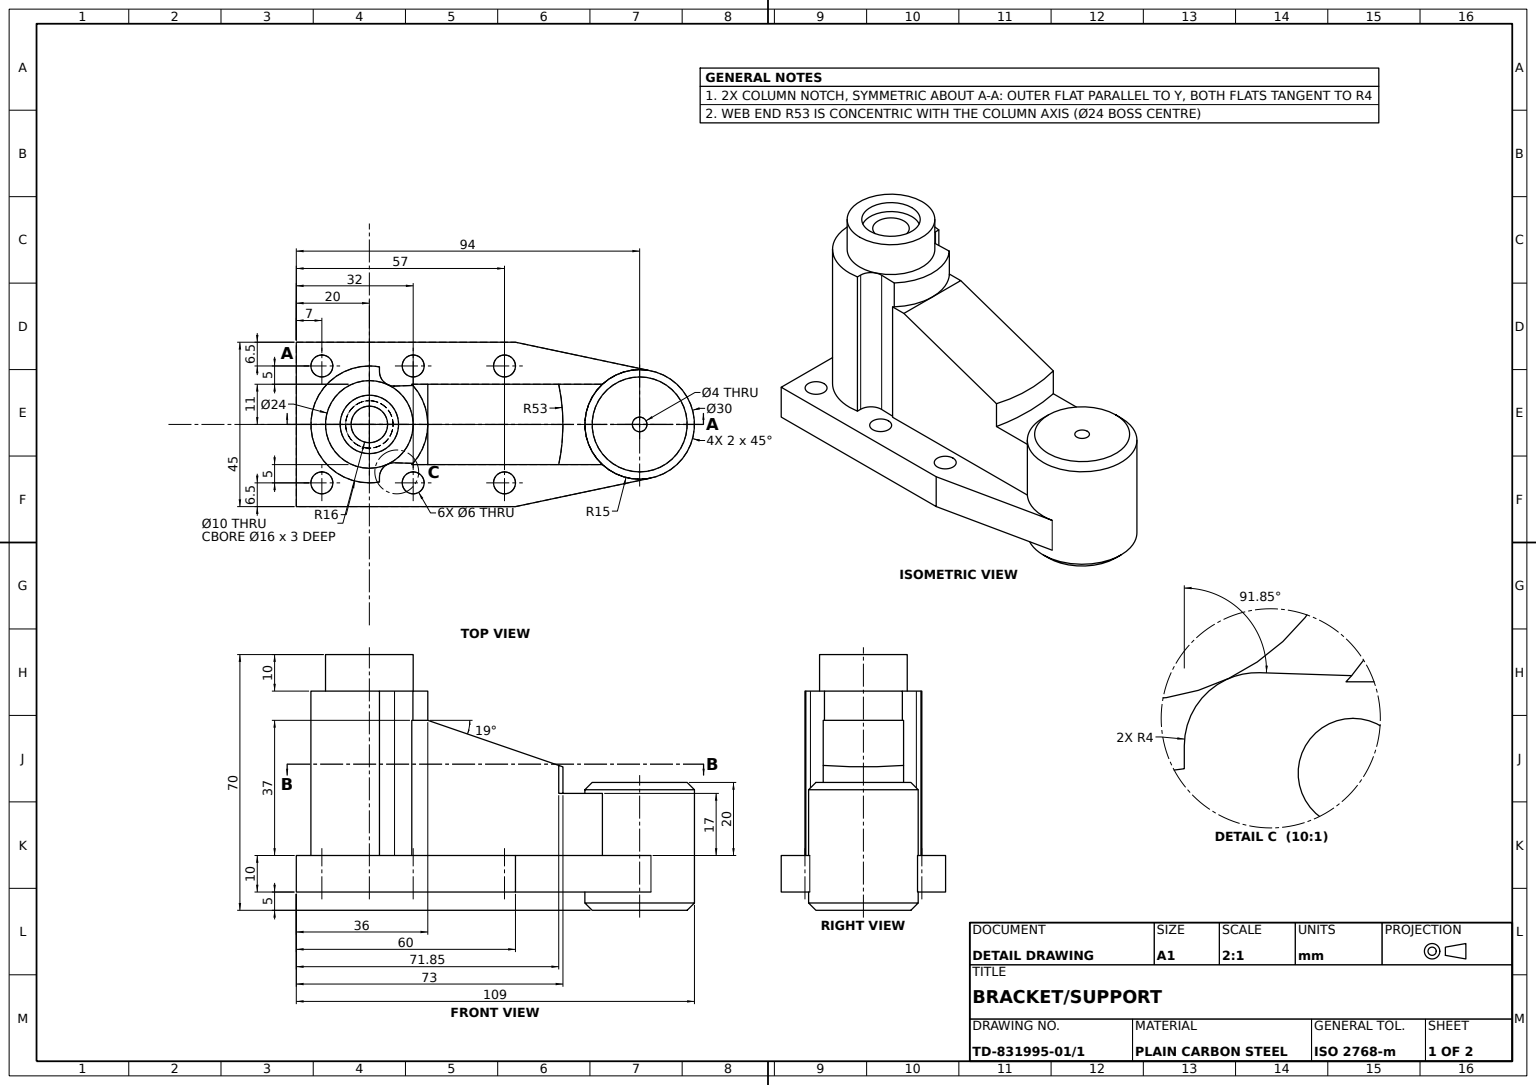
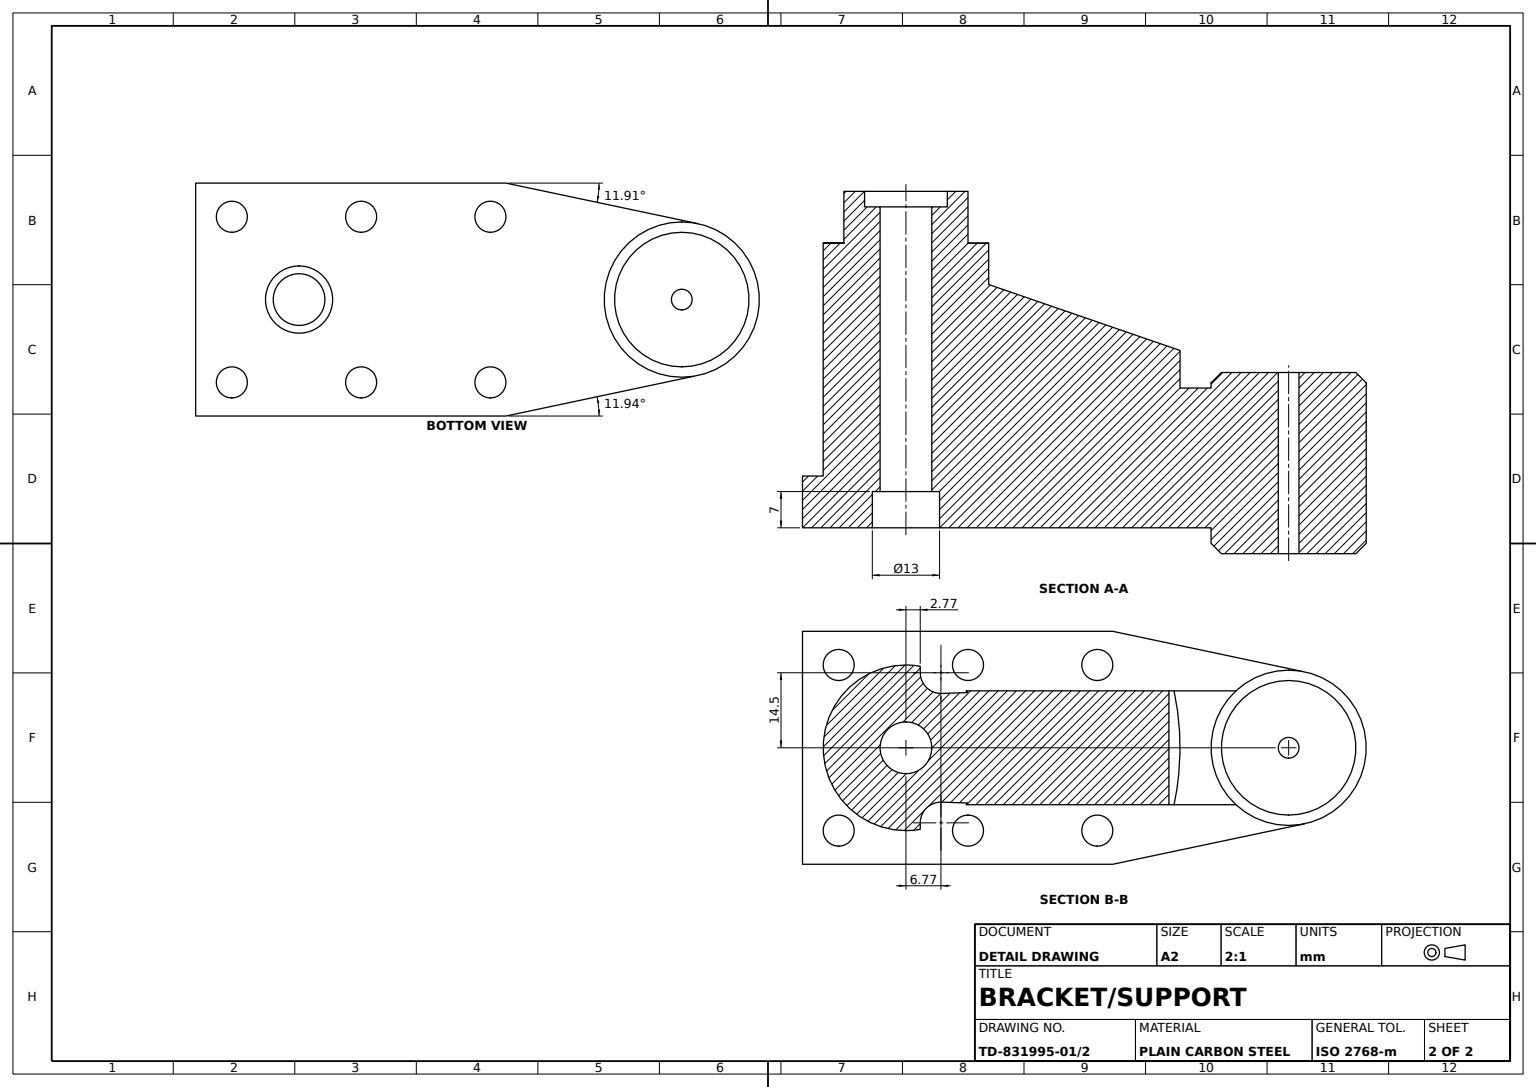
from build123d import *

# Parameters (mm, degrees)
PIVOT_HUB_SKETCH_R           = 15
PIVOT_HUB_30_DEPTH           = 35
BASE_PLATE_DEPTH             = 10
COLUMN_SKETCH_R              = 16
COLUMN_32_DEPTH              = 45
SLOPED_WEB_DEPTH             = 37
WEB_TRIM_CUT_DEPTH           = 37
WEB_PAD_DEPTH                = 17
HUB_CHAMFER_A_SIZE           = 2
HUB_CHAMFER_B_SIZE           = 2
HUB_PIN_HOLE_SKETCH_R        = 2
HUB_PIN_HOLE_4_DEPTH         = 39
COLUMN_TOP_BOSS_SKETCH_R     = 12
COLUMN_TOP_BOSS_24_DEPTH     = 10
TOP_COUNTERBORE_SKETCH_R     = 8
TOP_COUNTERBORE_16_DEPTH     = 3
COLUMN_BORE_SKETCH_R         = 5
COLUMN_BORE_10_DEPTH         = 106
BOTTOM_COUNTERBORE_SKETCH_R  = 6.5
BOTTOM_COUNTERBORE_13_DEPTH  = 7
COLUMN_START                 = -45
COLUMN_SLOT_DEPTH            = 45
BASE_MOUNTING_HOLES_SKETCH_R = 3
BASE_MOUNTING_HOLES_6_DEPTH  = 196


with BuildPart() as part:
    # Pivot Hub Sketch → Pivot Hub Ø30 (new body)
    with BuildSketch(Plane(origin=(0, 0, 0), x_dir=(1, 0, 0), z_dir=(0, 1, 0))):
        with Locations(Location((0, 0, 0), (0, 0, 270))):
            Circle(PIVOT_HUB_SKETCH_R)
    extrude(amount=PIVOT_HUB_30_DEPTH)

    # Base Plate Sketch → Base Plate (add)
    with BuildSketch(Plane(origin=(0, 5, 0), x_dir=(1, 0, 0), z_dir=(0, 1, 0))):
        with BuildLine():
            Line((-94, 0), (-94, 22.5))
            Line((-94, 22.5), (-34, 22.5))
            Line((-34, 22.5), (2.327936287, 14.81825606))
            ThreePointArc((2.327936287, 14.81825606), (-14.994927572, -0.390060375), (3.095195933, -14.677185089))
            Line((3.095195933, -14.677185089), (-34, -22.5))
            Line((-34, -22.5), (-94, -22.5))
            Line((-94, -22.5), (-94, 0))
        make_face()
    extrude(amount=BASE_PLATE_DEPTH)

    # Column Sketch → Column Ø32 (add)
    with BuildSketch(Plane(origin=(0, 15, 0), x_dir=(1, 0, 0), z_dir=(0, 1, 0))):
        with Locations(Location((-74, 0, 0), (0, 0, 90))):
            Circle(COLUMN_SKETCH_R)
    extrude(amount=COLUMN_32_DEPTH)

    # Web Sketch → Sloped Web (add)
    with BuildSketch(Plane(origin=(0, 15, 0), x_dir=(1, 0, 0), z_dir=(0, 1, 0))):
        with BuildLine():
            Line((-74, 11), (-22.154074413, 11))
            ThreePointArc((-22.154074413, 11), (-21, 0), (-22.154074413, -11))
            Line((-22.154074413, -11), (-74, -11))
            ThreePointArc((-74, -11), (-85, 0), (-74, 11))
        make_face()
    extrude(amount=SLOPED_WEB_DEPTH)

    # Web Trim Sketch → Web Trim Cut (cut)
    with BuildSketch(Plane.XY.offset(11)):
        Polygon((-58, 52), (-22.154074413, 52), (-16.501763131, 52), (-16.501763131, 37.711011143), align=None)
    extrude(amount=-WEB_TRIM_CUT_DEPTH, mode=Mode.SUBTRACT)

    # Web Pad Sketch → Web Pad (add)
    with BuildSketch(Plane(origin=(0, 15, 0), x_dir=(1, 0, 0), z_dir=(0, 1, 0))):
        with BuildLine():
            Line((-22.154074413, 11), (-1.869546507, 11))
            Line((-1.869546507, 11), (-1.869546507, -11))
            Line((-1.869546507, -11), (-22.154074413, -11))
            ThreePointArc((-22.154074413, -11), (-21, 0), (-22.154074413, 11))
        make_face()
    extrude(amount=WEB_PAD_DEPTH)

    # Hub Chamfer A
    hub_chamfer_a_edges = [part.edges().sort_by_distance(p)[0] for p in [
        (0, 35, -15),
    ]]
    chamfer(hub_chamfer_a_edges, length=HUB_CHAMFER_A_SIZE)

    # Hub Chamfer B
    hub_chamfer_b_edges = [part.edges().sort_by_distance(p)[0] for p in [
        (0, 0, -15),
    ]]
    chamfer(hub_chamfer_b_edges, length=HUB_CHAMFER_B_SIZE)

    # Hub Pin Hole Sketch → Hub Pin Hole Ø4 (cut)
    with BuildSketch(Plane(origin=(0, 35, 0), x_dir=(1, 0, 0), z_dir=(0, 1, 0))):
        with Locations(Location((0, 0, 0), (0, 0, 270))):
            Circle(HUB_PIN_HOLE_SKETCH_R)
    extrude(amount=-HUB_PIN_HOLE_4_DEPTH, mode=Mode.SUBTRACT)

    # Column Top Boss Sketch → Column Top Boss Ø24 (add)
    with BuildSketch(Plane(origin=(0, 60, 0), x_dir=(1, 0, 0), z_dir=(0, 1, 0))):
        with Locations(Location((-74, 0, 0), (0, 0, 270))):
            Circle(COLUMN_TOP_BOSS_SKETCH_R)
    extrude(amount=COLUMN_TOP_BOSS_24_DEPTH)

    # Top Counterbore Sketch → Top Counterbore Ø16 (cut)
    with BuildSketch(Plane(origin=(0, 70, 0), x_dir=(1, 0, 0), z_dir=(0, 1, 0))):
        with Locations(Location((-74, 0, 0), (0, 0, 270))):
            Circle(TOP_COUNTERBORE_SKETCH_R)
    extrude(amount=-TOP_COUNTERBORE_16_DEPTH, mode=Mode.SUBTRACT)

    # Column Bore Sketch → Column Bore Ø10 (cut)
    with BuildSketch(Plane(origin=(0, 67, 0), x_dir=(1, 0, 0), z_dir=(0, 1, 0))):
        with Locations(Location((-74, 0, 0), (0, 0, 270))):
            Circle(COLUMN_BORE_SKETCH_R)
    extrude(amount=-COLUMN_BORE_10_DEPTH, mode=Mode.SUBTRACT)

    # Bottom Counterbore Sketch → Bottom Counterbore Ø13 (cut)
    with BuildSketch(Plane.XZ.offset(-5)):
        with Locations(Location((-74, 0, 0), (0, 0, 270))):
            Circle(BOTTOM_COUNTERBORE_SKETCH_R)
    extrude(amount=-BOTTOM_COUNTERBORE_13_DEPTH, mode=Mode.SUBTRACT)

    # Column Slot Sketch → Column Slot (cut)
    with BuildSketch(Plane(origin=(0, 60, 0), x_dir=(1, 0, 0), z_dir=(0, 1, 0)).offset(COLUMN_START)):
        with BuildLine():
            ThreePointArc((-62.071178187, 10.663170736), (-66.223257294, 13.982927908), (-71.233832555, 15.759070965))
            Line((-71.233832555, 15.759070965), (-71.233832555, 14.49893024))
            ThreePointArc((-71.233832555, 14.49893024), (-70.680112836, 12.468375582), (-69.172256444, 11))
            ThreePointArc((-69.172256444, 11), (-69.049905074, 10.934960458), (-68.925374416, 10.87419768))
            ThreePointArc((-68.925374416, 10.87419768), (-68.037177922, 10.580431009), (-67.105038845, 10.501004255))
            Line((-67.105038845, 10.501004255), (-62.071178187, 10.663170736))
        make_face()
        with BuildLine():
            Line((-62.071178187, -10.663170736), (-67.105038845, -10.501004255))
            ThreePointArc((-67.105038845, -10.501004255), (-70.016351662, -11.62532842), (-71.233832555, -14.49893024))
            Line((-71.233832555, -14.49893024), (-71.233832555, -15.759070965))
            ThreePointArc((-71.233832555, -15.759070965), (-66.223257294, -13.982927908), (-62.071178187, -10.663170736))
        make_face()
    extrude(amount=COLUMN_SLOT_DEPTH, mode=Mode.SUBTRACT)

    # Base Mounting Holes Sketch → Base Mounting Holes Ø6 (cut)
    with BuildSketch(Plane(origin=(0, 15, 0), x_dir=(1, 0, 0), z_dir=(0, 1, 0))):
        with Locations(Location((-87, -16, 0), (0, 0, 270))):
            Circle(BASE_MOUNTING_HOLES_SKETCH_R)
        with Locations(Location((-62, -16, 0), (0, 0, 270))):
            Circle(BASE_MOUNTING_HOLES_SKETCH_R)
        with Locations(Location((-37, -16, 0), (0, 0, 270))):
            Circle(BASE_MOUNTING_HOLES_SKETCH_R)
        with Locations(Location((-87, 16, 0), (0, 0, 270))):
            Circle(BASE_MOUNTING_HOLES_SKETCH_R)
        with Locations(Location((-37, 16, 0), (0, 0, 270))):
            Circle(BASE_MOUNTING_HOLES_SKETCH_R)
        with Locations(Location((-62, 16, 0), (0, 0, 270))):
            Circle(BASE_MOUNTING_HOLES_SKETCH_R)
    extrude(amount=-BASE_MOUNTING_HOLES_6_DEPTH, mode=Mode.SUBTRACT)


solid = part.part
